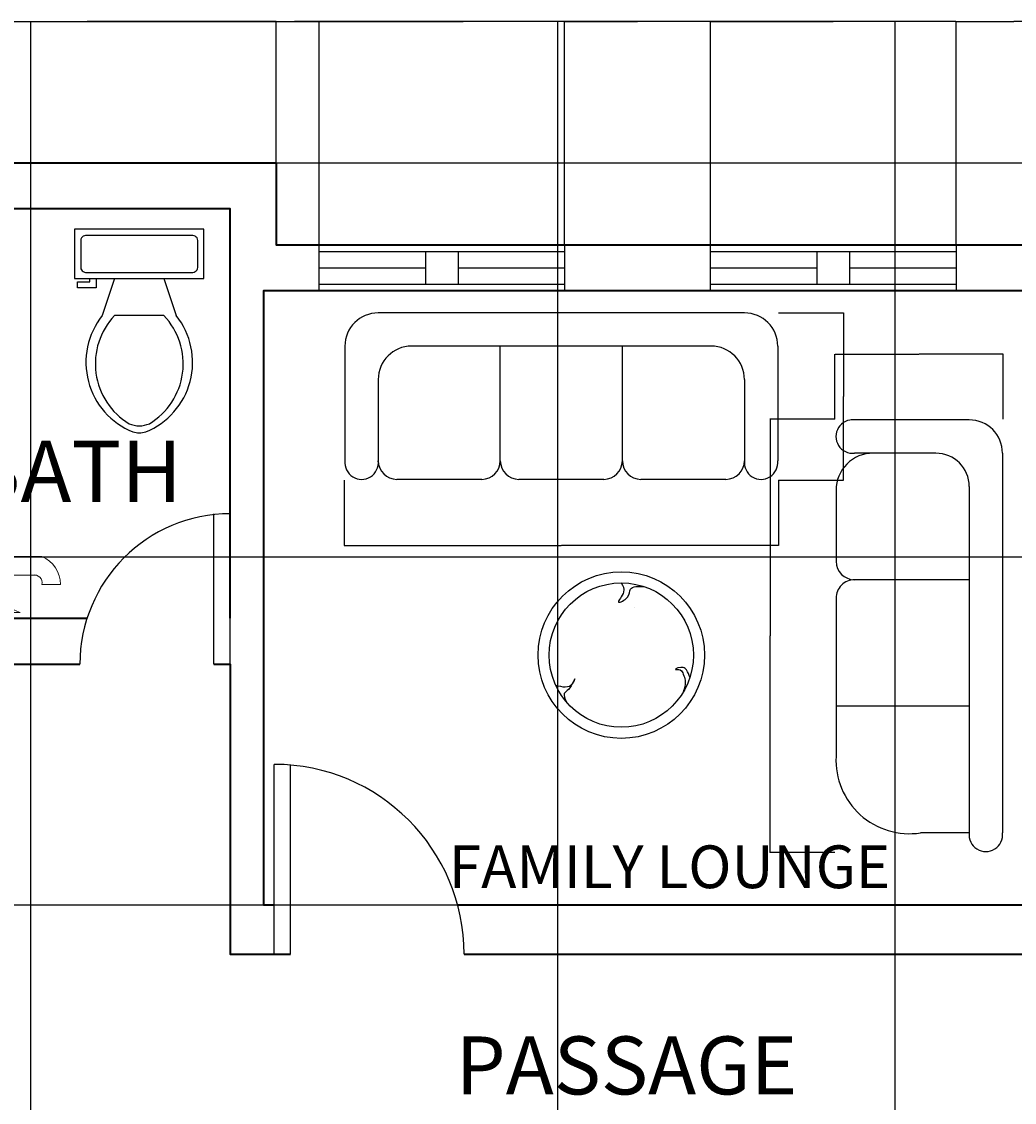
# Model space of a CAD drawing. Units: millimetres. Extents: x 19292 to 100733, y 12374 to 26974.
# Tile 21 of 24: x 47819 to 52672, y 18270 to 23551. Entities that reach past the tile are written whole.
import ezdxf

# ---------------------------------------------------------------- set-up
doc = ezdxf.new("R2010")
doc.units = ezdxf.units.MM
for name, color, linetype, lineweight in [('A-ANNO-DIMS', 2, 'Continuous', 18), ('A-AREA-IDEN', 3, 'Continuous', 25), ('A-DOOR', 4, 'Continuous', 25), ('A-FLOR-FIXT', 9, 'Continuous', 18), ('A-FURN', 8, 'Continuous', 18), ('A-GLAZ', 3, 'Continuous', 25), ('A-WALL', 7, 'Continuous', 35)]:
    doc.layers.add(name, color=color, linetype=linetype, lineweight=lineweight)
doc.layers.add('FURNITURE', color=40, linetype='Continuous')
doc.layers.add('WINDOWS', color=50, linetype='Continuous')
doc.styles.get("Standard").update_dxf_attribs({"font": 'arial.ttf'})
doc.dimstyles.get("Standard").update_dxf_attribs({"dimtxt": 0.18, "dimasz": 0.18, "dimexe": 0.18, "dimexo": 0.0625, "dimgap": 0.09, "dimtad": 0, "dimtih": 1, "dimtoh": 1, "dimdec": 4, "dimzin": 0, "dimdsep": 46, "dimtxsty": 'Standard', "dimcen": 0.09, "dimadec": 0, "dimazin": 0, "dimtfac": 1, "dimtdec": 4, "dimtofl": 0, "dimtmove": 0, "dimatfit": 3, "dimfxl": 1, "dimtolj": 1, "dimtzin": 0, "dimarcsym": 0})

# ---------------------------------------------------------------- blocks, each defined once
blk = doc.blocks.new('WC01')
at = {"layer": 'FURNITURE'}
for p, q in [((10.5, 0), (-10.5, 0)), ((-10.5, 0), (-10.5, -8)), ((10.5, -8), (10.5, 0)), ((8.5, -1), (-8.5, -1)), ((-9.5, -2), (-9.5, -6)), ((9.5, -6), (9.5, -2)), ((-8.5, -7), (8.5, -7)), ((-10.5, -8), (10.5, -8)), ((-10, -9.5), (-10, -8.5)), ((-10, -8.5), (-8, -8.5)), ((-8, -8.5), (-8, -8)), ((-7, -8), (-7, -9.5)), ((-4, -8), (-6, -14)), ((4, -8), (6, -14)), ((-7, -9.5), (-10, -9.5)), ((4, -14), (-4, -14))]:
    blk.add_line(p, q, dxfattribs=at)
for centre, radius, start, end in [((-8.62, -1.88), 0.884, 81.8699, 188.1301), ((8.62, -1.88), 0.884, 351.8699, 98.1301), ((-8.62, -6.12), 0.884, 171.8699, 278.1301), ((8.62, -6.12), 0.884, 261.8699, 8.1301), ((3.52, -21.58), 12.17, 141.4691, 247.9714), ((4.2, -21.82), 11.33, 136.3677, 238.9468), ((-3.52, -21.58), 12.17, 292.0284, 38.5307), ((-4.2, -21.82), 11.33, 301.053, 43.6321), ((0, -27.88), 4, 245.7318, 294.2682), ((0, -29), 4, 254.8605, 285.1395)]:
    blk.add_arc(centre, radius, start, end, dxfattribs=at)
blk = doc.blocks.new('TAP-SIDELEV')
for p, q in [((1, 4.25), (2, 4.25)), ((2, 3.75), (1, 3.75)), ((1.25, 3), (1.25, 3.5)), ((1.75, 3.5), (1.75, 3)), ((1, 3), (3.84, 3)), ((3.527, 2), (2, 2)), ((4.84, 1.5), (3.84, 1.5)), ((0, 0), (0.25, 0)), ((0.25, 0), (2.676, 0))]:
    blk.add_line(p, q)
for points in [[(1, 3.75), (1, 4.25)], [(1.25, 4.5), (1.75, 4.5)], [(2, 4.25), (2, 3.75)], [(1.75, 3.5), (1.25, 3.5)]]:
    blk.add_lwpolyline(points)
for centre, radius, start, end in [((1.242, 4.258), 0.243, 88.22243, 181.7776), ((1.757, 4.258), 0.243, 358.2224, 91.77757), ((1.242, 3.742), 0.243, 178.2224, 271.7776), ((1.757, 3.742), 0.243, 268.2224, 1.77757), ((5.084, -0.028), 5.084, 143.4467, 179.6834), ((3.172, 1.471), 1.668, 0.98277, 66.40494), ((2.377, 1.325), 0.773, 119.18009, 204.87157), ((3.434, 1.594), 0.417, 347.0192, 102.9808), ((3.051, 1.375), 1.425, 195.2551, 254.7449)]:
    blk.add_arc(centre, radius, start, end)
blk = doc.blocks.new('WW')
at = {"layer": 'WINDOWS'}
for p, q in [((-5183.9, -4940.9), (-3983.9, -4940.9)), ((-4663.9, -4940.9), (-4663.9, -5100.9)), ((-4503.9, -4940.9), (-4503.9, -5100.9)), ((-4503.9, -4940.9), (-4503.9, -5100.9)), ((-5183.9, -5020.9), (-4663.9, -5020.9)), ((-4503.9, -5020.9), (-3983.9, -5020.9)), ((-5183.9, -5100.9), (-3983.9, -5100.9))]:
    blk.add_line(p, q, dxfattribs=at)
for points in [[(-5183.9, -5133.4), (-5183.9, -4908.4)], [(-3983.9, -4908.4), (-3983.9, -5133.4)]]:
    blk.add_lwpolyline(points, dxfattribs=at)
blk = doc.blocks.new('3sofa')
at = {"layer": 'FURNITURE'}
for p, q in [((29.7, 0), (-29.7, 0)), ((-35.1, -5.4), (-35.1, -24)), ((24.3, -5.4), (-24.3, -5.4)), ((-9.9, -24), (-9.9, -5.4)), ((9.9, -24), (9.9, -5.4)), ((35.1, -5.4), (35.1, -24)), ((35.1, -5.4), (35.1, -24)), ((-29.7, -10.8), (-29.7, -24)), ((29.7, -10.8), (29.7, -24)), ((-12.9, -27), (-26.7, -27)), ((6.9, -27), (-6.9, -27)), ((26.7, -27), (12.9, -27))]:
    blk.add_line(p, q, dxfattribs=at)
for centre, radius, start, end in [((-29.7, -5.4), 5.4, 90, 180), ((29.7, -5.4), 5.4, 0, 90), ((-24.3, -10.8), 5.4, 90, 180), ((24.3, -10.8), 5.4, 0, 90), ((-32.4, -24.285), 2.715, 173.97442, 6.02558), ((-26.7, -24), 3, 180, 270), ((-12.9, -24), 3, 270, 0), ((-6.9, -24), 3, 180, 270), ((6.9, -24), 3, 270, 0), ((12.9, -24), 3, 180, 270), ((26.7, -24), 3, 270, 0), ((32.4, -24.285), 2.715, 173.97442, 6.02558)]:
    blk.add_arc(centre, radius, start, end, dxfattribs=at)
blk = doc.blocks.new('2sofa-hf')
at = {"layer": 'FURNITURE'}
for p, q in [((-27, -29.85), (-27, 31.72)), ((-21.6, -24.45), (-21.6, 31.72)), ((-21.6, 31.72), (-13.69, 31.72)), ((0, -6.32), (0, 19.35)), ((-21.62, 11.2), (-0.02, 11.2)), ((-21.57, -9.32), (-2.97, -9.32)), ((0, -23.85), (0, -12.32)), ((-16.2, -29.85), (-3, -29.85)), ((-21.6, -35.25), (-2.43, -35.25))]:
    blk.add_line(p, q, dxfattribs=at)
for centre, radius, start, end in [((-24.3, 32.03), 2.72, 353.479, 186.521), ((-11.92, 19.92), 11.93, 357.2261, 98.5207), ((-3, -6.32), 3, 270, 0), ((-3, -12.32), 3, 0, 90), ((-16.2, -24.45), 5.4, 180, 270), ((-6, -23.85), 6, 270, 0), ((-21.6, -29.85), 5.4, 180, 270), ((-2.71, -32.55), 2.72, 263.9744, 96.0256)]:
    blk.add_arc(centre, radius, start, end, dxfattribs=at)
blk = doc.blocks.new('PUFFY')
at = {"layer": 'FURNITURE', "const_width": 0.00005}
for points in [[(-1.711, 5.906, 1), (-1.698, 5.906, 1)], [(-1.249, 6.008, 1), (-1.237, 6.008, 1)], [(-0.429, 6.161, 1), (-0.417, 6.161, 1)], [(-2.787, 5.138, 1), (-2.774, 5.138, 1)], [(-2.479, 5.496, 1), (-2.467, 5.496, 1)], [(-2.428, 5.036, 1), (-2.416, 5.036, 1)], [(-1.916, 5.394, 1), (-1.903, 5.394, 1)], [(-1.864, 5.036, 1), (-1.852, 5.036, 1)], [(-1.147, 5.036, 1), (-1.134, 5.036, 1)], [(-0.891, 5.496, 1), (-0.878, 5.496, 1)], [(-0.276, 5.803, 1), (-0.263, 5.803, 1)], [(0.8, 5.036, 1), (0.813, 5.036, 1)], [(1.262, 5.803, 1), (1.274, 5.803, 1)], [(1.415, 5.343, 1), (1.428, 5.343, 1)], [(1.569, 4.933, 1), (1.582, 4.933, 1)], [(1.877, 5.547, 1), (1.889, 5.547, 1)], [(2.184, 4.882, 1), (2.197, 4.882, 1)], [(2.697, 5.547, 1), (2.709, 5.547, 1)], [(2.85, 4.933, 1), (2.863, 4.933, 1)], [(-2.479, 4.524, 1), (-2.467, 4.524, 1)], [(-1.659, 4.575, 1), (-1.647, 4.575, 1)], [(-1.198, 4.37, 1), (-1.186, 4.37, 1)], [(-0.686, 4.626, 1), (-0.673, 4.626, 1)], [(1.159, 4.319, 1), (1.172, 4.319, 1)], [(1.569, 4.421, 1), (1.582, 4.421, 1)], [(2.44, 4.268, 1), (2.453, 4.268, 1)], [(3.824, -1.464, 1), (3.837, -1.464, 1)], [(4.593, -1.822, 1), (4.606, -1.822, 1)], [(-3.453, -2.896, 1), (-3.441, -2.896, 1)], [(3.722, -2.538, 1), (3.734, -2.538, 1)], [(4.029, -2.129, 1), (4.042, -2.129, 1)], [(4.183, -2.896, 1), (4.196, -2.896, 1)], [(4.439, -2.692, 1), (4.452, -2.692, 1)], [(4.542, -2.231, 1), (4.554, -2.231, 1)], [(5.054, -2.026, 1), (5.067, -2.026, 1)], [(5.105, -2.487, 1), (5.118, -2.487, 1)], [(-4.786, -3.818, 1), (-4.773, -3.818, 1)], [(-4.581, -3.306, 1), (-4.568, -3.306, 1)], [(-4.068, -3.306, 1), (-4.056, -3.306, 1)], [(-3.709, -3.766, 1), (-3.697, -3.766, 1)], [(-3.094, -3.459, 1), (-3.082, -3.459, 1)], [(3.619, -3.05, 1), (3.632, -3.05, 1)], [(3.875, -3.562, 1), (3.888, -3.562, 1)], [(4.49, -3.459, 1), (4.503, -3.459, 1)], [(4.9, -3.05, 1), (4.913, -3.05, 1)], [(5.157, -3.664, 1), (5.169, -3.664, 1)], [(5.31, -3.204, 1), (5.323, -3.204, 1)], [(-4.324, -4.483, 1), (-4.312, -4.483, 1)], [(-4.222, -3.92, 1), (-4.209, -3.92, 1)], [(-3.914, -4.227, 1), (-3.902, -4.227, 1)], [(-3.453, -4.483, 1), (-3.441, -4.483, 1)], [(-3.197, -4.073, 1), (-3.184, -4.073, 1)], [(-2.736, -4.483, 1), (-2.723, -4.483, 1)], [(3.67, -4.329, 1), (3.683, -4.329, 1)], [(4.132, -4.278, 1), (4.144, -4.278, 1)], [(4.49, -3.971, 1), (4.503, -3.971, 1)], [(-3.812, -4.892, 1), (-3.799, -4.892, 1)], [(-3.146, -5.046, 1), (-3.133, -5.046, 1)], [(-2.531, -5.353, 1), (-2.518, -5.353, 1)]]:
    blk.add_lwpolyline(points, format="xyb", close=True, dxfattribs=at)
at = {"layer": 'FURNITURE'}
for radius in [7.5, 6.5]:
    blk.add_circle((0, 0), radius, dxfattribs=at)
for points, knots in [([(0, 6.5), (0.148, 6.243), (0.47, 5.685), (-0.715, 4.457), (0.771, 5.119), (0.69, 6.238), (1.526, 6.197), (2.042, 6.171)], [0, 0, 0, 0, 0.853207, 1.850764, 2.77014, 3.532386, 4.762324, 4.762324, 4.762324, 4.762324]), ([(6.187, -1.993), (6.093, -1.767), (5.955, -1.431), (5.557, -0.962), (4.503, -1.357), (5.424, -1.248), (5.598, -1.766), (5.859, -2.423), (5.689, -2.977), (5.577, -3.339)], [0, 0, 0, 0, 0.731037, 1.082325, 1.814636, 2.257188, 2.72894, 3.301273, 4.384204, 4.384204, 4.384204, 4.384204]), ([(-5.915, -2.694), (-5.318, -2.862), (-4.56, -3.069), (-4.022, -1.724), (-4.58, -3.096), (-5.312, -3.455), (-5.082, -3.934), (-4.946, -4.218)], [0.010289, 0.010289, 0.010289, 0.010289, 1.160744, 1.473738, 2.290002, 2.686083, 3.263094, 3.263094, 3.263094, 3.263094])]:
    blk.add_open_spline(points, degree=3, knots=knots, dxfattribs=at)
blk = doc.blocks.new('DOOR-750')
for p, q in [((655.3, 0), (655.3, 735.3)), ((735.3, 0), (735.3, 735.3)), ((735.3, 0), (655.3, 0)), ((735.3, 0), (655.3, 0))]:
    blk.add_line(p, q)
blk.add_arc((735.3, 0), 735.3, 90, 180)
blk = doc.blocks.new('*D42')
at = {"layer": 'A-ANNO-DIMS', "color": 0, "lineweight": -2, "transparency": 16777216}
for p, q in [((49396.3, 21310.2), (49396.3, 20991.8)), ((51518.1, 21310.2), (51518.1, 20991.8)), ((49396.4, 20991.9), (50455.7, 20991.9)), ((51518, 20991.9), (50458.7, 20991.9))]:
    blk.add_line(p, q, dxfattribs=at)
at = {"layer": 'A-ANNO-DIMS', "color": 0, "transparency": 16777216}
for points in [[(49396.4, 20992), (49396.4, 20991.9), (49396.3, 20991.9)], [(51518, 20992), (51518, 20991.9), (51518.1, 20991.9)]]:
    blk.add_solid(points, dxfattribs=at)
at = {"layer": 'Defpoints', "color": 0, "transparency": 16777216}
for p in [(49396.3, 21310.2), (51518.1, 21310.2), (51518.1, 20991.9)]:
    blk.add_point(p, dxfattribs=at)
at = {"layer": 'A-ANNO-DIMS', "color": 0, "transparency": 16777216, "insert": (50457.2, 20991.9), "char_height": 0.18, "attachment_point": 5}
blk.add_mtext('\\A1;3-SEAT SOFA 2122 TYP.', dxfattribs=at)
blk = doc.blocks.new('*D43')
at = {"layer": 'A-ANNO-DIMS', "color": 0, "lineweight": -2, "transparency": 16777216}
for p, q in [((51518.2, 22128), (51836.6, 22128)), ((51836.4, 22127.8), (51836.4, 21719.3)), ((51836.4, 21310.4), (51836.4, 21718.9)), ((51518.2, 21310.2), (51836.6, 21310.2))]:
    blk.add_line(p, q, dxfattribs=at)
at = {"layer": 'A-ANNO-DIMS', "color": 0, "transparency": 16777216}
for points in [[(51836.4, 22127.8), (51836.5, 22127.8), (51836.4, 22128)], [(51836.4, 21310.4), (51836.5, 21310.4), (51836.4, 21310.2)]]:
    blk.add_solid(points, dxfattribs=at)
at = {"layer": 'Defpoints', "color": 0, "transparency": 16777216}
for p in [(51518.1, 22128), (51836.4, 22128), (51518.1, 21310.2)]:
    blk.add_point(p, dxfattribs=at)
at = {"layer": 'A-ANNO-DIMS', "color": 0, "transparency": 16777216, "insert": (51836.4, 21719.1), "char_height": 0.18, "attachment_point": 5}
blk.add_mtext('\\A1;818 TYP.', dxfattribs=at)
blk = doc.blocks.new('*D44')
at = {"layer": 'A-ANNO-DIMS', "color": 0, "lineweight": -2, "transparency": 16777216}
for p, q in [((51794.8, 21608.2), (51477.2, 21608.2)), ((51477.4, 21608), (51477.4, 20550)), ((51477.4, 19491.6), (51477.4, 20549.7)), ((51794.8, 19491.5), (51477.2, 19491.5))]:
    blk.add_line(p, q, dxfattribs=at)
at = {"layer": 'A-ANNO-DIMS', "color": 0, "transparency": 16777216}
for points in [[(51477.3, 21608), (51477.4, 21608), (51477.4, 21608.2)], [(51477.3, 19491.6), (51477.4, 19491.6), (51477.4, 19491.5)]]:
    blk.add_solid(points, dxfattribs=at)
at = {"layer": 'Defpoints', "color": 0, "transparency": 16777216}
for p in [(51794.9, 21608.2), (51477.4, 19491.5), (51794.9, 19491.5)]:
    blk.add_point(p, dxfattribs=at)
at = {"layer": 'A-ANNO-DIMS', "color": 0, "transparency": 16777216, "insert": (51477.4, 20549.8), "char_height": 0.18, "attachment_point": 5}
blk.add_mtext('\\A1;2-SEAT SOFA 2117 TYP.', dxfattribs=at)
blk = doc.blocks.new('*D45')
at = {"layer": 'A-ANNO-DIMS', "color": 0, "lineweight": -2, "transparency": 16777216}
for p, q in [((51794.9, 21608.3), (51794.9, 21925.9)), ((51795.1, 21925.7), (52205.5, 21925.7)), ((52617.1, 21925.7), (52206.7, 21925.7)), ((52617.2, 21608.3), (52617.2, 21925.9))]:
    blk.add_line(p, q, dxfattribs=at)
at = {"layer": 'A-ANNO-DIMS', "color": 0, "transparency": 16777216}
for points in [[(51795.1, 21925.8), (51795.1, 21925.7), (51794.9, 21925.7)], [(52617.1, 21925.8), (52617.1, 21925.7), (52617.2, 21925.7)]]:
    blk.add_solid(points, dxfattribs=at)
at = {"layer": 'Defpoints', "color": 0, "transparency": 16777216}
for p in [(51794.9, 21925.7), (51794.9, 21608.2), (52617.2, 21608.2)]:
    blk.add_point(p, dxfattribs=at)
at = {"layer": 'A-ANNO-DIMS', "color": 0, "transparency": 16777216, "insert": (52206.1, 21925.7), "char_height": 0.18, "attachment_point": 5}
blk.add_mtext('\\A1;822 TYP.', dxfattribs=at)
blk = doc.blocks.new('*D93')
at = {"layer": 'A-ANNO-DIMS', "color": 0, "lineweight": -2, "transparency": 16777216}
for p, q in [((47214, 22635.8), (47214, 23550.9)), ((47214.2, 23550.7), (48138.6, 23550.7)), ((49063.8, 23550.7), (48139.3, 23550.7)), ((49064, 22860.8), (49064, 23550.9))]:
    blk.add_line(p, q, dxfattribs=at)
at = {"layer": 'A-ANNO-DIMS', "color": 0, "transparency": 16777216}
for points in [[(47214.2, 23550.8), (47214.2, 23550.7), (47214, 23550.7)], [(49063.8, 23550.8), (49063.8, 23550.7), (49064, 23550.7)]]:
    blk.add_solid(points, dxfattribs=at)
at = {"layer": 'Defpoints', "color": 0, "transparency": 16777216}
for p in [(49064, 23550.7), (49064, 22860.7), (47214, 22635.7)]:
    blk.add_point(p, dxfattribs=at)
at = {"layer": 'A-ANNO-DIMS', "color": 0, "transparency": 16777216, "insert": (48139, 23550.7), "char_height": 0.18, "attachment_point": 5}
blk.add_mtext('\\A1;1850', dxfattribs=at)
blk = doc.blocks.new('*D94')
at = {"layer": 'A-ANNO-DIMS', "color": 0, "lineweight": -2, "transparency": 16777216}
for p, q in [((49064, 22460.8), (49064, 23550.9)), ((49064.2, 23550.7), (49167.9, 23550.7)), ((49272.6, 23550.7), (49168.8, 23550.7)), ((49272.7, 22460.8), (49272.7, 23550.9))]:
    blk.add_line(p, q, dxfattribs=at)
at = {"layer": 'A-ANNO-DIMS', "color": 0, "transparency": 16777216}
for points in [[(49064.2, 23550.8), (49064.2, 23550.7), (49064, 23550.7)], [(49272.6, 23550.8), (49272.6, 23550.7), (49272.7, 23550.7)]]:
    blk.add_solid(points, dxfattribs=at)
at = {"layer": 'Defpoints', "color": 0, "transparency": 16777216}
for p in [(49272.7, 23550.7), (49064, 22460.7), (49272.7, 22460.7)]:
    blk.add_point(p, dxfattribs=at)
at = {"layer": 'A-ANNO-DIMS', "color": 0, "transparency": 16777216, "insert": (49168.4, 23550.7), "char_height": 0.18, "attachment_point": 5}
blk.add_mtext('\\A1;208.74', dxfattribs=at)
blk = doc.blocks.new('*D95')
at = {"layer": 'A-ANNO-DIMS', "color": 0, "lineweight": -2, "transparency": 16777216}
for p, q in [((49272.7, 22460.8), (49272.7, 23550.9)), ((49272.9, 23550.7), (49872.4, 23550.7)), ((50472.6, 23550.7), (49873.1, 23550.7)), ((50472.7, 22460.8), (50472.7, 23550.9))]:
    blk.add_line(p, q, dxfattribs=at)
at = {"layer": 'A-ANNO-DIMS', "color": 0, "transparency": 16777216}
for points in [[(49272.9, 23550.8), (49272.9, 23550.7), (49272.7, 23550.7)], [(50472.6, 23550.8), (50472.6, 23550.7), (50472.7, 23550.7)]]:
    blk.add_solid(points, dxfattribs=at)
at = {"layer": 'Defpoints', "color": 0, "transparency": 16777216}
for p in [(50472.7, 23550.7), (49272.7, 22460.7), (50472.7, 22460.7)]:
    blk.add_point(p, dxfattribs=at)
at = {"layer": 'A-ANNO-DIMS', "color": 0, "transparency": 16777216, "insert": (49872.7, 23550.7), "char_height": 0.18, "attachment_point": 5}
blk.add_mtext('\\A1;1200', dxfattribs=at)
blk = doc.blocks.new('*D96')
at = {"layer": 'A-ANNO-DIMS', "color": 0, "lineweight": -2, "transparency": 16777216}
for p, q in [((50472.7, 22460.8), (50472.7, 23550.9)), ((50472.9, 23550.7), (50829.2, 23550.7)), ((51186.3, 23550.7), (50830, 23550.7)), ((51186.5, 22460.8), (51186.5, 23550.9))]:
    blk.add_line(p, q, dxfattribs=at)
at = {"layer": 'A-ANNO-DIMS', "color": 0, "transparency": 16777216}
for points in [[(50472.9, 23550.8), (50472.9, 23550.7), (50472.7, 23550.7)], [(51186.3, 23550.8), (51186.3, 23550.7), (51186.5, 23550.7)]]:
    blk.add_solid(points, dxfattribs=at)
at = {"layer": 'Defpoints', "color": 0, "transparency": 16777216}
for p in [(51186.5, 23550.7), (50472.7, 22460.7), (51186.5, 22460.7)]:
    blk.add_point(p, dxfattribs=at)
at = {"layer": 'A-ANNO-DIMS', "color": 0, "transparency": 16777216, "insert": (50829.6, 23550.7), "char_height": 0.18, "attachment_point": 5}
blk.add_mtext('\\A1;713.8', dxfattribs=at)
blk = doc.blocks.new('*D97')
at = {"layer": 'A-ANNO-DIMS', "color": 0, "lineweight": -2, "transparency": 16777216}
for p, q in [((51186.5, 22460.8), (51186.5, 23550.9)), ((51186.7, 23550.7), (51786.2, 23550.7)), ((52386.3, 23550.7), (51786.9, 23550.7)), ((52386.5, 22460.8), (52386.5, 23550.9))]:
    blk.add_line(p, q, dxfattribs=at)
at = {"layer": 'A-ANNO-DIMS', "color": 0, "transparency": 16777216}
for points in [[(51186.7, 23550.8), (51186.7, 23550.7), (51186.5, 23550.7)], [(52386.3, 23550.8), (52386.3, 23550.7), (52386.5, 23550.7)]]:
    blk.add_solid(points, dxfattribs=at)
at = {"layer": 'Defpoints', "color": 0, "transparency": 16777216}
for p in [(52386.5, 23550.7), (51186.5, 22460.7), (52386.5, 22460.7)]:
    blk.add_point(p, dxfattribs=at)
at = {"layer": 'A-ANNO-DIMS', "color": 0, "transparency": 16777216, "insert": (51786.5, 23550.7), "char_height": 0.18, "attachment_point": 5}
blk.add_mtext('\\A1;1200', dxfattribs=at)
blk = doc.blocks.new('*D98')
at = {"layer": 'A-ANNO-DIMS', "color": 0, "lineweight": -2, "transparency": 16777216}
for p, q in [((52386.5, 22460.8), (52386.5, 23550.9)), ((52386.7, 23550.7), (52668.7, 23550.7)), ((52951.3, 23550.7), (52669.3, 23550.7)), ((52951.5, 22460.8), (52951.5, 23550.9))]:
    blk.add_line(p, q, dxfattribs=at)
at = {"layer": 'A-ANNO-DIMS', "color": 0, "transparency": 16777216}
for points in [[(52386.7, 23550.8), (52386.7, 23550.7), (52386.5, 23550.7)], [(52951.3, 23550.8), (52951.3, 23550.7), (52951.5, 23550.7)]]:
    blk.add_solid(points, dxfattribs=at)
at = {"layer": 'Defpoints', "color": 0, "transparency": 16777216}
for p in [(52951.5, 23550.7), (52386.5, 22460.7), (52951.5, 22460.7)]:
    blk.add_point(p, dxfattribs=at)
at = {"layer": 'A-ANNO-DIMS', "color": 0, "transparency": 16777216, "insert": (52669, 23550.7), "char_height": 0.18, "attachment_point": 5}
blk.add_mtext('\\A1;565', dxfattribs=at)
blk = doc.blocks.new('*D102')
at = {"layer": 'A-ANNO-DIMS', "color": 0, "lineweight": -2, "transparency": 16777216}
for p, q in [((43614.1, 20935.7), (57530.2, 20935.7)), ((57530, 20935.5), (57530, 20085.9)), ((57530, 19235.9), (57530, 20085.5)), ((43614.1, 19235.7), (57530.2, 19235.7))]:
    blk.add_line(p, q, dxfattribs=at)
at = {"layer": 'A-ANNO-DIMS', "color": 0, "transparency": 16777216}
for points in [[(57530, 20935.5), (57530.1, 20935.5), (57530, 20935.7)], [(57530, 19235.9), (57530.1, 19235.9), (57530, 19235.7)]]:
    blk.add_solid(points, dxfattribs=at)
at = {"layer": 'Defpoints', "color": 0, "transparency": 16777216}
for p in [(43614, 20935.7), (43614, 19235.7), (57530, 19235.7)]:
    blk.add_point(p, dxfattribs=at)
at = {"layer": 'A-ANNO-DIMS', "color": 0, "transparency": 16777216, "insert": (57530, 20085.7), "char_height": 0.18, "attachment_point": 5}
blk.add_mtext('\\A1;1700', dxfattribs=at)
blk = doc.blocks.new('*D111')
at = {"layer": 'A-ANNO-DIMS', "color": 0, "lineweight": -2, "transparency": 16777216}
for p, q in [((49064.1, 22860.7), (57530.2, 22860.7)), ((57530, 22860.5), (57530, 22660.9)), ((57530, 22460.9), (57530, 22660.5)), ((56839.3, 22460.7), (57530.2, 22460.7))]:
    blk.add_line(p, q, dxfattribs=at)
at = {"layer": 'A-ANNO-DIMS', "color": 0, "transparency": 16777216}
for points in [[(57530, 22860.5), (57530.1, 22860.5), (57530, 22860.7)], [(57530, 22460.9), (57530.1, 22460.9), (57530, 22460.7)]]:
    blk.add_solid(points, dxfattribs=at)
at = {"layer": 'Defpoints', "color": 0, "transparency": 16777216}
for p in [(49064, 22860.7), (57530, 22860.7), (56839.2, 22460.7)]:
    blk.add_point(p, dxfattribs=at)
at = {"layer": 'A-ANNO-DIMS', "color": 0, "transparency": 16777216, "insert": (57530, 22660.7), "char_height": 0.18, "attachment_point": 5}
blk.add_mtext('\\A1;400', dxfattribs=at)
blk = doc.blocks.new('*D112')
at = {"layer": 'A-ANNO-DIMS', "color": 0, "lineweight": -2, "transparency": 16777216}
for p, q in [((43389, 22860.7), (43389, 12813.8)), ((56840, 15985.7), (56840, 12813.8)), ((43389.2, 12814), (50114.1, 12814)), ((56839.9, 12814), (50114.9, 12814))]:
    blk.add_line(p, q, dxfattribs=at)
at = {"layer": 'A-ANNO-DIMS', "color": 0, "transparency": 16777216}
for points in [[(43389.2, 12814), (43389.2, 12814), (43389, 12814)], [(56839.9, 12814), (56839.9, 12814), (56840, 12814)]]:
    blk.add_solid(points, dxfattribs=at)
at = {"layer": 'Defpoints', "color": 0, "transparency": 16777216}
for p in [(43389, 22860.7), (56840, 15985.7), (56840, 12814)]:
    blk.add_point(p, dxfattribs=at)
at = {"layer": 'A-ANNO-DIMS', "color": 0, "transparency": 16777216, "insert": (50114.5, 12814), "char_height": 0.18, "attachment_point": 5}
blk.add_mtext('\\A1;13451', dxfattribs=at)
blk = doc.blocks.new('*D116')
at = {"layer": 'A-ANNO-DIMS', "color": 0, "lineweight": -2, "transparency": 16777216}
for p, q in [((47864.5, 13544.1), (47864.5, 23550.9)), ((47864.7, 23550.7), (49976.7, 23550.7)), ((52089.5, 23550.7), (49977.5, 23550.7)), ((52089.7, 13544.1), (52089.7, 23550.9))]:
    blk.add_line(p, q, dxfattribs=at)
at = {"layer": 'A-ANNO-DIMS', "color": 0, "transparency": 16777216}
for points in [[(47864.7, 23550.8), (47864.7, 23550.7), (47864.5, 23550.7)], [(52089.5, 23550.8), (52089.5, 23550.7), (52089.7, 23550.7)]]:
    blk.add_solid(points, dxfattribs=at)
at = {"layer": 'Defpoints', "color": 0, "transparency": 16777216}
for p in [(52089.7, 23550.7), (47864.5, 13544), (52089.7, 13544)]:
    blk.add_point(p, dxfattribs=at)
at = {"layer": 'A-ANNO-DIMS', "color": 0, "transparency": 16777216, "insert": (49977.1, 23550.7), "char_height": 0.18, "attachment_point": 5}
blk.add_mtext('\\A1;4225', dxfattribs=at)
blk = doc.blocks.new('*D119')
at = {"layer": 'A-ANNO-DIMS', "color": 0, "lineweight": -2, "transparency": 16777216}
for p, q in [((47864.5, 15131.5), (47864.5, 23550.9)), ((47864.7, 23550.7), (49151.7, 23550.7)), ((50439.3, 23550.7), (49152.4, 23550.7)), ((50439.5, 15131.5), (50439.5, 23550.9))]:
    blk.add_line(p, q, dxfattribs=at)
at = {"layer": 'A-ANNO-DIMS', "color": 0, "transparency": 16777216}
for points in [[(47864.7, 23550.8), (47864.7, 23550.7), (47864.5, 23550.7)], [(50439.3, 23550.8), (50439.3, 23550.7), (50439.5, 23550.7)]]:
    blk.add_solid(points, dxfattribs=at)
at = {"layer": 'Defpoints', "color": 0, "transparency": 16777216}
for p in [(50439.5, 23550.7), (47864.5, 15131.4), (50439.5, 15131.4)]:
    blk.add_point(p, dxfattribs=at)
at = {"layer": 'A-ANNO-DIMS', "color": 0, "transparency": 16777216, "insert": (49152, 23550.7), "char_height": 0.18, "attachment_point": 5}
blk.add_mtext('\\A1;2575', dxfattribs=at)

msp = doc.modelspace()

# ---------------------------------------------------------------- linework, layer by layer
at = {"layer": 'A-DOOR'}
for p, q in [((49053.956, 18993.993), (49053.956, 19921.691)), ((49053.956, 18993.993), (49053.956, 19921.691)), ((49133.956, 18993.993), (49133.956, 19921.691)), ((49053.956, 18993.993), (49133.956, 18993.993)), ((49053.956, 18993.993), (49133.956, 18993.993))]:
    msp.add_line(p, q, dxfattribs=at)
msp.add_arc((49053.956, 18993.993), 927.699, 0, 90, dxfattribs=at)
at = {"layer": 'A-WALL'}
for points in [[(43388.992, 22860.725), (49063.992, 22860.725), (49063.992, 22460.725), (56838.992, 22460.725), (56840.043, 15985.725), (54414.519, 15985.331), (54414.519, 14906.403), (52089.658, 14906.403), (52089.658, 13543.993), (44043.674, 13543.993), (44026.778, 19012.695), (43388.992, 19010.725), (43388.992, 22860.725)], [(48838.992, 20635.725), (48838.992, 22635.725), (47438.992, 22635.725), (47438.992, 20635.725), (48138.992, 20635.725)], [(52726.51, 22183.986), (52726.51, 22235.725), (49001.51, 22235.725), (49001.51, 19235.725), (49053.956, 19235.725)], [(49949.607, 19235.725), (52726.51, 19235.725), (52726.51, 21336.287)], [(47438.992, 20163.424), (47438.992, 20410.725), (48103.72, 20410.725)], [(48758.992, 20410.725), (48838.992, 20410.725), (48838.992, 18993.993), (49133.956, 18993.993)], [(49981.654, 18993.993), (52726.51, 18993.993), (52726.51, 18855.887)]]:
    msp.add_lwpolyline(points, dxfattribs=at)

# ---------------------------------------------------------------- block references
at = {"layer": 'A-DOOR'}
msp.add_blockref('DOOR-750', (48103.72, 20410.725), dxfattribs=at)
at = {"layer": 'A-FLOR-FIXT'}
for name, p, xscale, yscale, zscale in [('WC01', (48394.002, 22536.306), 30.13269765108242, 30.13269765108242, 30.13269765108242), ('TAP-SIDELEV', (47568.669, 20664.116), 91.03318940714036, 91.03318940714036, 91.03318940714036)]:
    msp.add_blockref(name, p, dxfattribs=dict(at, xscale=xscale, yscale=yscale, zscale=zscale))
at = {"layer": 'A-FURN'}
for name, p, xscale, yscale, zscale in [('3sofa', (50457.202, 22127.955), 30.13269765108242, 30.13269765108242, 30.13269765108242), ('PUFFY', (50750.31, 20455.662), 54.24717212198793, 54.24717212198793, 54.24717212198793)]:
    msp.add_blockref(name, p, dxfattribs=dict(at, xscale=xscale, yscale=yscale, zscale=zscale))
at = {"layer": 'A-FURN', "xscale": 30.13269765108242, "yscale": 30.13269765108242, "zscale": 30.13269765108242, "rotation": 180}
msp.add_blockref('2sofa-hf', (51800.09, 20542.781), dxfattribs=at)
at = {"layer": 'A-GLAZ'}
for p in [(54456.602, 27369.102), (56370.378, 27369.102)]:
    msp.add_blockref('WW', p, dxfattribs=at)

# ---------------------------------------------------------------- texts
at = {"layer": 'A-AREA-IDEN'}
for s, height, p in [('BATH', 299.1707, (47545.657, 21204.251)), ('FAMILY LOUNGE', 208.87112, (49907.481, 19316.848)), ('PASSAGE', 283.3894, (49940.566, 18308.997))]:
    msp.add_text(s, height=height, dxfattribs=at).set_placement(p)

# ---------------------------------------------------------------- dimensions: what is measured, and where the dimension line sits
at = {"layer": 'A-ANNO-DIMS'}
for base, p1, p2, override, picture, middle in [((49063.992, 23550.725), (47213.992, 22635.725), (49063.992, 22860.725), {"dimdec": 0, "dimlfac": 1, "dimrnd": 0, "dimzin": 0, "dimdsep": 46, "dimlunit": 2}, '*D93', (48138.992, 23550.725)), ((52089.658, 23550.725), (47864.519, 13543.993), (52089.658, 13543.993), {"dimdec": 0, "dimlfac": 1, "dimrnd": 0, "dimzin": 0, "dimdsep": 46, "dimlunit": 2}, '*D116', (49977.089, 23550.725)), ((50439.519, 23550.725), (47864.519, 15131.403), (50439.519, 15131.403), {"dimdec": 0, "dimlfac": 1, "dimrnd": 0, "dimzin": 0, "dimdsep": 46, "dimlunit": 2}, '*D119', (49152.019, 23550.725)), ((49272.734, 23550.725), (49063.992, 22460.725), (49272.734, 22460.725), {"dimdec": 2, "dimlfac": 1, "dimrnd": 0, "dimzin": 0, "dimdsep": 46, "dimlunit": 2}, '*D94', (49168.363, 23550.725)), ((50472.734, 23550.725), (49272.734, 22460.725), (50472.734, 22460.725), {"dimdec": 0, "dimlfac": 1, "dimrnd": 0, "dimzin": 0, "dimdsep": 46, "dimlunit": 2}, '*D95', (49872.734, 23550.725)), ((51186.51, 23550.725), (50472.734, 22460.725), (51186.51, 22460.725), {"dimdec": 1, "dimlfac": 1, "dimrnd": 0, "dimzin": 0, "dimdsep": 46, "dimlunit": 2}, '*D96', (50829.622, 23550.725)), ((52386.51, 23550.725), (51186.51, 22460.725), (52386.51, 22460.725), {"dimdec": 0, "dimlfac": 1, "dimrnd": 0, "dimzin": 0, "dimdsep": 46, "dimlunit": 2}, '*D97', (51786.51, 23550.725)), ((52951.492, 23550.725), (52386.51, 22460.725), (52951.492, 22460.725), {"dimdec": 0, "dimlfac": 1, "dimrnd": 0, "dimzin": 0, "dimdsep": 46, "dimlunit": 2}, '*D98', (52669.001, 23550.725)), ((56840.043, 12813.993), (43388.992, 22860.725), (56840.043, 15985.725), {"dimdec": 0, "dimlfac": 1, "dimrnd": 0, "dimzin": 0, "dimdsep": 46, "dimlunit": 2}, '*D112', (50114.517, 12813.993))]:
    dim = msp.add_linear_dim(base=base, p1=p1, p2=p2, dimstyle='Standard', override=override, dxfattribs=at)
    dim.commit()
    dim.dimension.update_dxf_attribs({"geometry": picture, "text_midpoint": middle})
for base, p1, p2, picture, middle in [((57530.043, 22860.725), (56839.196, 22460.725), (49063.992, 22860.725), '*D111', (57530.043, 22660.725)), ((57530.043, 19235.725), (43613.992, 20935.725), (43613.992, 19235.725), '*D102', (57530.043, 20085.725))]:
    dim = msp.add_linear_dim(base=base, p1=p1, p2=p2, angle=90, dimstyle='Standard', override={"dimdec": 0, "dimlfac": 1, "dimrnd": 0, "dimzin": 0, "dimdsep": 46, "dimlunit": 2}, dxfattribs=at)
    dim.commit()
    dim.dimension.update_dxf_attribs({"geometry": picture, "text_midpoint": middle})
for base, p1, p2, angle, text, picture, middle in [((51836.426, 22127.955), (51518.144, 21310.227), (51518.144, 22127.955), 90, '<> TYP.', '*D43', (51836.426, 21719.091)), ((51794.878, 21925.739), (52617.249, 21608.225), (51794.878, 21608.225), 180, '<> TYP.', '*D45', (52206.064, 21925.739)), ((51477.363, 19491.46), (51794.878, 21608.225), (51794.878, 19491.46), 270, '2-SEAT SOFA <> TYP.', '*D44', (51477.363, 20549.842))]:
    dim = msp.add_linear_dim(base=base, p1=p1, p2=p2, angle=angle, text=text, dimstyle='Standard', override={"dimdec": 0, "dimrnd": 0, "dimzin": 0, "dimlunit": 2}, dxfattribs=at)
    dim.commit()
    dim.dimension.update_dxf_attribs({"geometry": picture, "text_midpoint": middle})
dim = msp.add_linear_dim(base=(51518.144, 20991.944), p1=(49396.26, 21310.227), p2=(51518.144, 21310.227), text='3-SEAT SOFA <> TYP.', dimstyle='Standard', override={"dimdec": 0, "dimrnd": 0, "dimzin": 0, "dimlunit": 2}, dxfattribs=at)
dim.commit()
dim.dimension.update_dxf_attribs({"geometry": '*D42', "text_midpoint": (50457.202, 20991.944)})

doc.saveas('drawing.dxf')
